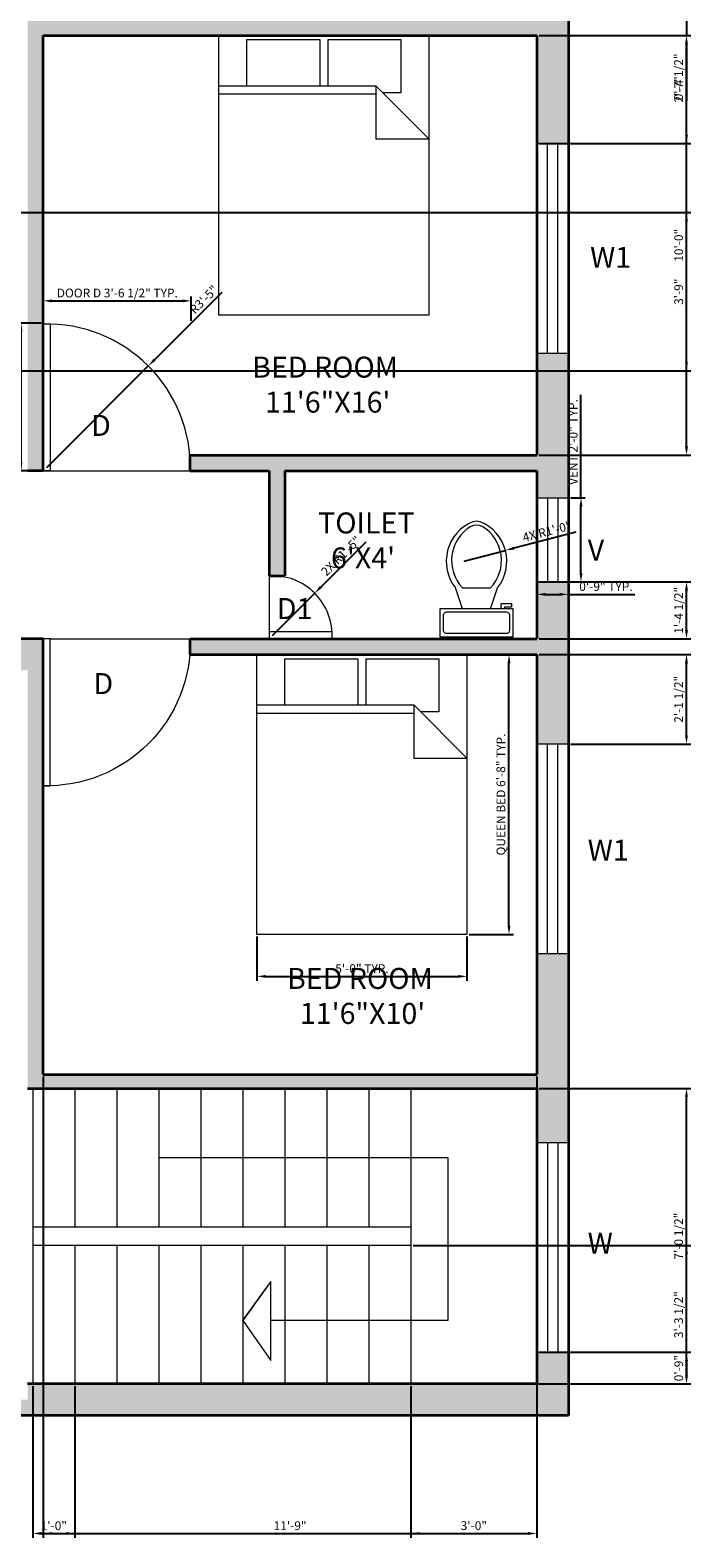
# Model space of a CAD drawing. Units: inches. Extents: x 5030 to 5465, y 5339 to 6047.
# Tile 2 of 5: x 5275 to 5465, y 5340 to 5771. Entities that reach past the tile are written whole.
import ezdxf

# ---------------------------------------------------------------- set-up
doc = ezdxf.new("R2010")
doc.units = ezdxf.units.IN
for name, color, linetype, lineweight in [('A-ANNO-DIMS', 2, 'Continuous', 18), ('A-ANNO-TEXT', 7, 'Continuous', 18), ('A-AREA-IDEN', 7, 'Continuous', 25), ('A-DOOR', 3, 'Continuous', 18), ('A-FLOR-FIXT', 9, 'Continuous', 18), ('A-FLOR-STRS', 7, 'Continuous', 18), ('A-FURN', 8, 'Continuous', 18), ('A-GLAZ', 4, 'Continuous', 18), ('A-WALL', 7, 'Continuous', 35)]:
    doc.layers.add(name, color=color, linetype=linetype, lineweight=lineweight)
doc.layers.add('A-WALL-PATT', color=149, linetype='Continuous', lineweight=13, true_color=0x444546)
doc.styles.get("Standard").update_dxf_attribs({"font": 'arial.ttf'})
doc.dimstyles.new('ISO-25', dxfattribs={"dimtxt": 2.5, "dimasz": 2.5, "dimexe": 1.25, "dimexo": 0.625, "dimtad": 1, "dimlunit": 3, "dimtxsty": 'Standard', "dimcen": 2.5, "dimadec": 0, "dimazin": 0, "dimtfac": 1, "dimtmove": 0, "dimatfit": 3, "dimfxl": 1, "dimarcsym": 0})

# ---------------------------------------------------------------- blocks, each defined once
blk = doc.blocks.new('Bed - Queen')
for p, q in [((0, -80.00003), (0, 0)), ((0, 0), (59.99999, 0)), ((59.99999, 0), (59.99999, -80.00003)), ((7.99999, -1.2), (28.79998, -1.2)), ((7.99999, -14.4), (7.99999, -1.2)), ((28.79998, -1.2), (28.79998, -14.4)), ((31.19999, -1.2), (51.99999, -1.2)), ((31.19999, -14.4), (31.19999, -1.2)), ((51.99999, -1.2), (51.99999, -16.4)), ((0, -14.4), (44.8, -14.4)), ((44.8, -16.8), (0, -16.8)), ((59.99999, -29.6), (44.8, -14.4)), ((44.8, -14.4), (44.8, -29.6)), ((51.99999, -16.4), (46.79936, -16.4)), ((44.8, -29.6), (59.99999, -29.6)), ((59.99999, -80.00003), (0, -80.00003))]:
    blk.add_line(p, q)
blk = doc.blocks.new('Toilet - top')
for p, q in [((9.5, -6), (9.5, -2)), ((-10, -8.5), (-8, -8.5)), ((-10, -9.5), (-10, -8.5)), ((-8, -8.5), (-8, -8)), ((-7, -8), (-7, -9.5)), ((-4, -8), (-6, -14)), ((4, -8), (6, -14)), ((-7, -9.5), (-10, -9.5)), ((4, -14), (-4, -14))]:
    blk.add_line(p, q)
blk.add_lwpolyline([(10.5, -8), (10.5, 0), (-10.5, 0), (-10.5, -8)], close=True)
for points in [[(-9.5, -2), (-9.5, -6)], [(8.5, -1), (-8.5, -1)], [(-8.5, -7), (8.5, -7)]]:
    blk.add_lwpolyline(points)
for centre, radius, start, end in [((-8.62, -1.88), 0.884, 81.8699, 188.1301), ((8.62, -1.88), 0.884, 351.8699, 98.1301), ((-8.62, -6.12), 0.884, 171.8699, 278.1301), ((8.62, -6.12), 0.884, 261.8699, 8.1301), ((3.52, -21.58), 12.17, 141.4691, 247.9714), ((4.2, -21.82), 11.33, 136.3677, 238.9468), ((-3.52, -21.58), 12.17, 292.0284, 38.5307), ((-4.2, -21.82), 11.33, 301.053, 43.6321), ((0, -27.88), 4, 245.7318, 294.2682), ((0, -29), 4, 254.8605, 285.1395)]:
    blk.add_arc(centre, radius, start, end)
blk = doc.blocks.new('WIN-60IN')
for p, q in [((0, 60), (9, 60)), ((3, 60), (3, 0)), ((6, 60), (6, 0)), ((0, 0), (9, 0))]:
    blk.add_line(p, q)
blk = doc.blocks.new('VENT-24IN')
for p, q in [((0, 24), (9, 24)), ((3, 24), (3, 0)), ((6, 24), (6, 0)), ((0, 0), (9, 0))]:
    blk.add_line(p, q)
blk = doc.blocks.new('DOOR-SWING-42IN')
for p, q in [((0, 0), (0, 42)), ((0, 42), (2, 42)), ((2, 42), (2, 0)), ((2, 0), (0, 0))]:
    blk.add_line(p, q)
blk.add_arc((1, 1), 41.01, 358.6028, 91.3972)
blk = doc.blocks.new('DOOR-SWING-18IN')
for p, q in [((0, 18), (0, 2)), ((18, 2), (0, 2)), ((0, 2), (0, 0)), ((0, 0), (18, 0)), ((18, 0), (18, 2))]:
    blk.add_line(p, q)
blk.add_arc((1, 1), 17.03, 356.6335, 93.3665)
blk = doc.blocks.new('*D15')
at = {"layer": 'A-ANNO-DIMS', "color": 0, "lineweight": -2, "transparency": 16777216}
for p, q in [((5400.91, 5592), (5413.53, 5592)), ((5412.28, 5514.5), (5412.28, 5589.5)), ((5400.91, 5512), (5413.53, 5512))]:
    blk.add_line(p, q, dxfattribs=at)
at = {"layer": 'A-ANNO-DIMS', "color": 0, "transparency": 16777216}
for points in [[(5411.87, 5589.5), (5412.7, 5589.5), (5412.28, 5592)], [(5411.87, 5514.5), (5412.7, 5514.5), (5412.28, 5512)]]:
    blk.add_solid(points, dxfattribs=at)
at = {"layer": 'Defpoints', "color": 0, "transparency": 16777216}
for p in [(5400.28, 5592), (5412.28, 5592), (5400.28, 5512)]:
    blk.add_point(p, dxfattribs=at)
at = {"layer": 'A-ANNO-DIMS', "color": 0, "transparency": 16777216, "insert": (5410.29, 5552), "char_height": 2.5, "attachment_point": 5, "rotation": 90}
blk.add_mtext('QUEEN BED 6\'-8" TYP.', dxfattribs=at)
blk = doc.blocks.new('*D16')
at = {"layer": 'A-ANNO-DIMS', "color": 0, "lineweight": -2, "transparency": 16777216}
for p, q in [((5340.28, 5511.38), (5340.28, 5498.75)), ((5400.28, 5511.38), (5400.28, 5498.75)), ((5342.78, 5500), (5397.78, 5500))]:
    blk.add_line(p, q, dxfattribs=at)
at = {"layer": 'A-ANNO-DIMS', "color": 0, "transparency": 16777216}
for points in [[(5342.78, 5500.42), (5342.78, 5499.59), (5340.28, 5500)], [(5397.78, 5500.42), (5397.78, 5499.59), (5400.28, 5500)]]:
    blk.add_solid(points, dxfattribs=at)
at = {"layer": 'Defpoints', "color": 0, "transparency": 16777216}
for p in [(5340.28, 5512), (5400.28, 5512), (5400.28, 5500)]:
    blk.add_point(p, dxfattribs=at)
at = {"layer": 'A-ANNO-DIMS', "color": 0, "transparency": 16777216, "insert": (5370.28, 5501.9), "char_height": 2.5, "attachment_point": 5}
blk.add_mtext('5\'-0" TYP.', dxfattribs=at)
blk = doc.blocks.new('*D17')
at = {"layer": 'A-ANNO-DIMS', "color": 0, "lineweight": -2, "transparency": 16777216}
for p, q in [((5279.24, 5687.4), (5279.24, 5694.37)), ((5321.51, 5687.4), (5321.51, 5694.37)), ((5281.74, 5693.12), (5319.01, 5693.12))]:
    blk.add_line(p, q, dxfattribs=at)
at = {"layer": 'A-ANNO-DIMS', "color": 0, "transparency": 16777216}
for points in [[(5281.74, 5693.53), (5281.74, 5692.7), (5279.24, 5693.12)], [(5319.01, 5693.53), (5319.01, 5692.7), (5321.51, 5693.12)]]:
    blk.add_solid(points, dxfattribs=at)
at = {"layer": 'Defpoints', "color": 0, "transparency": 16777216}
for p in [(5321.51, 5693.12), (5279.24, 5686.78), (5321.51, 5686.78)]:
    blk.add_point(p, dxfattribs=at)
at = {"layer": 'A-ANNO-DIMS', "color": 0, "transparency": 16777216, "insert": (5300.38, 5695.04), "char_height": 2.5, "attachment_point": 5}
blk.add_mtext('DOOR D 3\'-6 1/2" TYP.', dxfattribs=at)
blk = doc.blocks.new('*D18')
at = {"layer": 'A-ANNO-DIMS', "color": 0, "lineweight": -2, "transparency": 16777216}
for p, q in [((5278.62, 5686.78), (5271.65, 5686.78)), ((5272.9, 5647), (5272.9, 5684.28)), ((5278.62, 5644.5), (5271.65, 5644.5))]:
    blk.add_line(p, q, dxfattribs=at)
at = {"layer": 'A-ANNO-DIMS', "color": 0, "transparency": 16777216}
for points in [[(5272.48, 5684.28), (5273.32, 5684.28), (5272.9, 5686.78)], [(5272.48, 5647), (5273.32, 5647), (5272.9, 5644.5)]]:
    blk.add_solid(points, dxfattribs=at)
at = {"layer": 'Defpoints', "color": 0, "transparency": 16777216}
for p in [(5272.9, 5686.78), (5279.24, 5686.78), (5279.24, 5644.5)]:
    blk.add_point(p, dxfattribs=at)
at = {"layer": 'A-ANNO-DIMS', "color": 0, "transparency": 16777216, "insert": (5270.98, 5665.64), "char_height": 2.5, "attachment_point": 5, "rotation": 90}
blk.add_mtext('3\'-6 1/2" TYP.', dxfattribs=at)
blk = doc.blocks.new('*D23')
at = {"layer": 'A-ANNO-DIMS', "color": 0, "lineweight": -2, "transparency": 16777216}
for p, q in [((5432.84, 5636.81), (5432.84, 5666.21)), ((5429.87, 5636.81), (5434.09, 5636.81)), ((5432.84, 5615.31), (5432.84, 5634.31)), ((5429.87, 5612.81), (5434.09, 5612.81))]:
    blk.add_line(p, q, dxfattribs=at)
at = {"layer": 'A-ANNO-DIMS', "color": 0, "transparency": 16777216}
for points in [[(5432.42, 5634.31), (5433.26, 5634.31), (5432.84, 5636.81)], [(5432.42, 5615.31), (5433.26, 5615.31), (5432.84, 5612.81)]]:
    blk.add_solid(points, dxfattribs=at)
at = {"layer": 'Defpoints', "color": 0, "transparency": 16777216}
for p in [(5429.24, 5636.81), (5432.84, 5636.81), (5429.24, 5612.81)]:
    blk.add_point(p, dxfattribs=at)
at = {"layer": 'A-ANNO-DIMS', "color": 0, "transparency": 16777216, "insert": (5430.94, 5652.76), "char_height": 2.5, "attachment_point": 5, "rotation": 90}
blk.add_mtext('VENT 2\'-0" TYP.', dxfattribs=at)
blk = doc.blocks.new('*D24')
at = {"layer": 'A-ANNO-DIMS', "color": 0, "lineweight": -2, "transparency": 16777216}
for p, q in [((5420.24, 5612.18), (5420.24, 5607.96)), ((5429.24, 5612.18), (5429.24, 5607.96)), ((5422.74, 5609.21), (5426.74, 5609.21)), ((5429.24, 5609.21), (5448.23, 5609.21))]:
    blk.add_line(p, q, dxfattribs=at)
at = {"layer": 'A-ANNO-DIMS', "color": 0, "transparency": 16777216}
for points in [[(5422.74, 5609.62), (5422.74, 5608.79), (5420.24, 5609.21)], [(5426.74, 5609.62), (5426.74, 5608.79), (5429.24, 5609.21)]]:
    blk.add_solid(points, dxfattribs=at)
at = {"layer": 'Defpoints', "color": 0, "transparency": 16777216}
for p in [(5420.24, 5612.81), (5429.24, 5612.81), (5429.24, 5609.21)]:
    blk.add_point(p, dxfattribs=at)
at = {"layer": 'A-ANNO-DIMS', "color": 0, "transparency": 16777216, "insert": (5439.98, 5611.11), "char_height": 2.5, "attachment_point": 5}
blk.add_mtext('0\'-9" TYP.', dxfattribs=at)
blk = doc.blocks.new('*D36')
at = {"layer": 'A-ANNO-DIMS', "color": 0, "lineweight": -2, "transparency": 16777216}
for p, q in [((5279.24, 5471.38), (5279.24, 5339.5)), ((5420.24, 5471.38), (5420.24, 5339.5)), ((5281.74, 5340.75), (5417.74, 5340.75))]:
    blk.add_line(p, q, dxfattribs=at)
at = {"layer": 'A-ANNO-DIMS', "color": 0, "transparency": 16777216}
for points in [[(5281.74, 5341.17), (5281.74, 5340.34), (5279.24, 5340.75)], [(5417.74, 5341.17), (5417.74, 5340.34), (5420.24, 5340.75)]]:
    blk.add_solid(points, dxfattribs=at)
at = {"layer": 'Defpoints', "color": 0, "transparency": 16777216}
for p in [(5279.24, 5472), (5420.24, 5472), (5420.24, 5340.75)]:
    blk.add_point(p, dxfattribs=at)
at = {"layer": 'A-ANNO-DIMS', "color": 0, "transparency": 16777216, "insert": (5349.74, 5342.65), "char_height": 2.5, "attachment_point": 5}
blk.add_mtext('11\'-9"', dxfattribs=at)
blk = doc.blocks.new('*D37')
at = {"layer": 'A-ANNO-DIMS', "color": 0, "lineweight": -2, "transparency": 16777216}
for p, q in [((5420.87, 5769), (5464.24, 5769)), ((5462.99, 5651.5), (5462.99, 5766.5)), ((5420.87, 5649), (5464.24, 5649))]:
    blk.add_line(p, q, dxfattribs=at)
at = {"layer": 'A-ANNO-DIMS', "color": 0, "transparency": 16777216}
for points in [[(5462.57, 5766.5), (5463.41, 5766.5), (5462.99, 5769)], [(5462.57, 5651.5), (5463.41, 5651.5), (5462.99, 5649)]]:
    blk.add_solid(points, dxfattribs=at)
at = {"layer": 'Defpoints', "color": 0, "transparency": 16777216}
for p in [(5420.24, 5769), (5462.99, 5769), (5420.24, 5649)]:
    blk.add_point(p, dxfattribs=at)
at = {"layer": 'A-ANNO-DIMS', "color": 0, "transparency": 16777216, "insert": (5461.09, 5709), "char_height": 2.5, "attachment_point": 5, "rotation": 90}
blk.add_mtext('10\'-0"', dxfattribs=at)
blk = doc.blocks.new('*D39')
at = {"layer": 'A-ANNO-DIMS', "color": 0, "lineweight": -2, "transparency": 16777216}
for p, q in [((5420.87, 5468), (5464.24, 5468)), ((5462.99, 5386), (5462.99, 5465.5)), ((5420.87, 5383.5), (5464.24, 5383.5))]:
    blk.add_line(p, q, dxfattribs=at)
at = {"layer": 'A-ANNO-DIMS', "color": 0, "transparency": 16777216}
for points in [[(5462.57, 5465.5), (5463.41, 5465.5), (5462.99, 5468)], [(5462.57, 5386), (5463.41, 5386), (5462.99, 5383.5)]]:
    blk.add_solid(points, dxfattribs=at)
at = {"layer": 'Defpoints', "color": 0, "transparency": 16777216}
for p in [(5420.24, 5468), (5462.99, 5468), (5420.24, 5383.5)]:
    blk.add_point(p, dxfattribs=at)
at = {"layer": 'A-ANNO-DIMS', "color": 0, "transparency": 16777216, "insert": (5461.07, 5425.75), "char_height": 2.5, "attachment_point": 5, "rotation": 90}
blk.add_mtext('7\'-0 1/2"', dxfattribs=at)
blk = doc.blocks.new('*D40')
at = {"layer": 'A-ANNO-DIMS', "color": 0, "lineweight": -2, "transparency": 16777216}
for p, q in [((5276.24, 5382.88), (5276.24, 5339.5)), ((5288.24, 5382.88), (5288.24, 5339.5)), ((5278.74, 5340.75), (5285.74, 5340.75))]:
    blk.add_line(p, q, dxfattribs=at)
at = {"layer": 'A-ANNO-DIMS', "color": 0, "transparency": 16777216}
for points in [[(5278.74, 5341.17), (5278.74, 5340.34), (5276.24, 5340.75)], [(5285.74, 5341.17), (5285.74, 5340.34), (5288.24, 5340.75)]]:
    blk.add_solid(points, dxfattribs=at)
at = {"layer": 'Defpoints', "color": 0, "transparency": 16777216}
for p in [(5276.24, 5383.5), (5288.24, 5383.5), (5288.24, 5340.75)]:
    blk.add_point(p, dxfattribs=at)
at = {"layer": 'A-ANNO-DIMS', "color": 0, "transparency": 16777216, "insert": (5282.24, 5342.65), "char_height": 2.5, "attachment_point": 5}
blk.add_mtext('1\'-0"', dxfattribs=at)
blk = doc.blocks.new('*D41')
at = {"layer": 'A-ANNO-DIMS', "color": 0, "lineweight": -2, "transparency": 16777216}
for p, q in [((5384.87, 5423.1), (5464.24, 5423.1)), ((5462.99, 5386), (5462.99, 5420.6)), ((5384.87, 5383.5), (5464.24, 5383.5))]:
    blk.add_line(p, q, dxfattribs=at)
at = {"layer": 'A-ANNO-DIMS', "color": 0, "transparency": 16777216}
for points in [[(5462.57, 5420.6), (5463.41, 5420.6), (5462.99, 5423.1)], [(5462.57, 5386), (5463.41, 5386), (5462.99, 5383.5)]]:
    blk.add_solid(points, dxfattribs=at)
at = {"layer": 'Defpoints', "color": 0, "transparency": 16777216}
for p in [(5384.24, 5423.1), (5462.99, 5423.1), (5384.24, 5383.5)]:
    blk.add_point(p, dxfattribs=at)
at = {"layer": 'A-ANNO-DIMS', "color": 0, "transparency": 16777216, "insert": (5461.07, 5403.3), "char_height": 2.5, "attachment_point": 5, "rotation": 90}
blk.add_mtext('3\'-3 1/2"', dxfattribs=at)
blk = doc.blocks.new('*D44')
at = {"layer": 'A-ANNO-DIMS', "color": 0, "lineweight": -2, "transparency": 16777216}
for p, q in [((5420.87, 5769), (5464.24, 5769)), ((5462.99, 5740.6), (5462.99, 5766.5)), ((5420.87, 5738.1), (5464.24, 5738.1))]:
    blk.add_line(p, q, dxfattribs=at)
at = {"layer": 'A-ANNO-DIMS', "color": 0, "transparency": 16777216}
for points in [[(5462.57, 5766.5), (5463.41, 5766.5), (5462.99, 5769)], [(5462.57, 5740.6), (5463.41, 5740.6), (5462.99, 5738.1)]]:
    blk.add_solid(points, dxfattribs=at)
at = {"layer": 'Defpoints', "color": 0, "transparency": 16777216}
for p in [(5420.24, 5769), (5462.99, 5769), (5420.24, 5738.1)]:
    blk.add_point(p, dxfattribs=at)
at = {"layer": 'A-ANNO-DIMS', "color": 0, "transparency": 16777216, "insert": (5461.11, 5753.55), "char_height": 2.5, "attachment_point": 5, "rotation": 90}
blk.add_mtext('2\'-7"', dxfattribs=at)
blk = doc.blocks.new('*D45')
at = {"layer": 'A-ANNO-DIMS', "color": 0, "lineweight": -2, "transparency": 16777216}
for p, q in [((5420.87, 5592), (5464.24, 5592)), ((5462.99, 5568.93), (5462.99, 5589.5)), ((5429.87, 5566.43), (5464.24, 5566.43))]:
    blk.add_line(p, q, dxfattribs=at)
at = {"layer": 'A-ANNO-DIMS', "color": 0, "transparency": 16777216}
for points in [[(5462.57, 5589.5), (5463.41, 5589.5), (5462.99, 5592)], [(5462.57, 5568.93), (5463.41, 5568.93), (5462.99, 5566.43)]]:
    blk.add_solid(points, dxfattribs=at)
at = {"layer": 'Defpoints', "color": 0, "transparency": 16777216}
for p in [(5420.24, 5592), (5462.99, 5592), (5429.24, 5566.43)]:
    blk.add_point(p, dxfattribs=at)
at = {"layer": 'A-ANNO-DIMS', "color": 0, "transparency": 16777216, "insert": (5461.07, 5579.22), "char_height": 2.5, "attachment_point": 5, "rotation": 90}
blk.add_mtext('2\'-1 1/2"', dxfattribs=at)
blk = doc.blocks.new('*D46')
at = {"layer": 'A-ANNO-DIMS', "color": 0, "lineweight": -2, "transparency": 16777216}
for p, q in [((5420.87, 5392.54), (5464.24, 5392.54)), ((5462.99, 5390.04), (5462.99, 5386)), ((5420.87, 5383.5), (5464.24, 5383.5))]:
    blk.add_line(p, q, dxfattribs=at)
at = {"layer": 'A-ANNO-DIMS', "color": 0, "transparency": 16777216}
for points in [[(5462.57, 5390.04), (5463.41, 5390.04), (5462.99, 5392.54)], [(5462.57, 5386), (5463.41, 5386), (5462.99, 5383.5)]]:
    blk.add_solid(points, dxfattribs=at)
at = {"layer": 'Defpoints', "color": 0, "transparency": 16777216}
for p in [(5420.24, 5392.54), (5420.24, 5383.5), (5462.99, 5383.5)]:
    blk.add_point(p, dxfattribs=at)
at = {"layer": 'A-ANNO-DIMS', "color": 0, "transparency": 16777216, "insert": (5461.09, 5388.02), "char_height": 2.5, "attachment_point": 5, "rotation": 90}
blk.add_mtext('0\'-9"', dxfattribs=at)
blk = doc.blocks.new('*D51')
at = {"layer": 'A-ANNO-DIMS', "color": 0, "lineweight": -2, "transparency": 16777216}
for p, q in [((5420.87, 5612.81), (5464.24, 5612.81)), ((5462.99, 5599), (5462.99, 5610.31)), ((5420.87, 5596.5), (5464.24, 5596.5))]:
    blk.add_line(p, q, dxfattribs=at)
at = {"layer": 'A-ANNO-DIMS', "color": 0, "transparency": 16777216}
for points in [[(5462.57, 5610.31), (5463.41, 5610.31), (5462.99, 5612.81)], [(5462.57, 5599), (5463.41, 5599), (5462.99, 5596.5)]]:
    blk.add_solid(points, dxfattribs=at)
at = {"layer": 'Defpoints', "color": 0, "transparency": 16777216}
for p in [(5420.24, 5612.81), (5462.99, 5612.81), (5420.24, 5596.5)]:
    blk.add_point(p, dxfattribs=at)
at = {"layer": 'A-ANNO-DIMS', "color": 0, "transparency": 16777216, "insert": (5461.07, 5604.66), "char_height": 2.5, "attachment_point": 5, "rotation": 90}
blk.add_mtext('1\'-4 1/2"', dxfattribs=at)
blk = doc.blocks.new('*D59')
at = {"layer": 'A-ANNO-DIMS', "color": 0, "lineweight": -2, "transparency": 16777216}
for p, q in [((5173.08, 5718.33), (5464.24, 5718.33)), ((5462.99, 5675.62), (5462.99, 5715.83)), ((5173.08, 5673.12), (5464.24, 5673.12))]:
    blk.add_line(p, q, dxfattribs=at)
at = {"layer": 'A-ANNO-DIMS', "color": 0, "transparency": 16777216}
for points in [[(5462.57, 5715.83), (5463.41, 5715.83), (5462.99, 5718.33)], [(5462.57, 5675.62), (5463.41, 5675.62), (5462.99, 5673.12)]]:
    blk.add_solid(points, dxfattribs=at)
at = {"layer": 'Defpoints', "color": 0, "transparency": 16777216}
for p in [(5172.45, 5718.33), (5462.99, 5718.33), (5172.45, 5673.12)]:
    blk.add_point(p, dxfattribs=at)
at = {"layer": 'A-ANNO-DIMS', "color": 0, "transparency": 16777216, "insert": (5461.09, 5695.72), "char_height": 2.5, "attachment_point": 5, "rotation": 90}
blk.add_mtext('3\'-9"', dxfattribs=at)
blk = doc.blocks.new('*D61')
at = {"layer": 'A-ANNO-DIMS', "color": 0, "lineweight": -2, "transparency": 16777216}
for p, q in [((5384.24, 5382.88), (5384.24, 5339.5)), ((5420.24, 5382.88), (5420.24, 5339.5)), ((5386.74, 5340.75), (5417.74, 5340.75))]:
    blk.add_line(p, q, dxfattribs=at)
at = {"layer": 'A-ANNO-DIMS', "color": 0, "transparency": 16777216}
for points in [[(5386.74, 5341.17), (5386.74, 5340.34), (5384.24, 5340.75)], [(5417.74, 5341.17), (5417.74, 5340.34), (5420.24, 5340.75)]]:
    blk.add_solid(points, dxfattribs=at)
at = {"layer": 'Defpoints', "color": 0, "transparency": 16777216}
for p in [(5384.24, 5383.5), (5420.24, 5383.5), (5420.24, 5340.75)]:
    blk.add_point(p, dxfattribs=at)
at = {"layer": 'A-ANNO-DIMS', "color": 0, "transparency": 16777216, "insert": (5402.24, 5342.66), "char_height": 2.5, "attachment_point": 5}
blk.add_mtext('3\'-0"', dxfattribs=at)
blk = doc.blocks.new('*D62')
at = {"layer": 'A-ANNO-DIMS', "color": 0, "lineweight": -2, "transparency": 16777216}
for p, q in [((5462.99, 5776), (5462.99, 5778.5)), ((5420.87, 5773.5), (5464.24, 5773.5)), ((5462.99, 5773.5), (5462.99, 5769)), ((5420.87, 5769), (5464.24, 5769)), ((5462.99, 5766.5), (5462.99, 5750.28))]:
    blk.add_line(p, q, dxfattribs=at)
at = {"layer": 'A-ANNO-DIMS', "color": 0, "transparency": 16777216}
for points in [[(5462.57, 5776), (5463.41, 5776), (5462.99, 5773.5)], [(5462.57, 5766.5), (5463.41, 5766.5), (5462.99, 5769)]]:
    blk.add_solid(points, dxfattribs=at)
at = {"layer": 'Defpoints', "color": 0, "transparency": 16777216}
for p in [(5420.24, 5773.5), (5420.24, 5769), (5462.99, 5769)]:
    blk.add_point(p, dxfattribs=at)
at = {"layer": 'A-ANNO-DIMS', "color": 0, "transparency": 16777216, "insert": (5461.07, 5757.14), "char_height": 2.5, "attachment_point": 5, "rotation": 90}
blk.add_mtext('0\'-4 1/2"', dxfattribs=at)
blk = doc.blocks.new('*D64')
at = {"layer": 'A-ANNO-DIMS', "color": 0, "lineweight": -2, "transparency": 16777216}
for p, q in [((5330.28, 5695.54), (5311.01, 5676.27)), ((5280.24, 5645.5), (5309.24, 5674.5))]:
    blk.add_line(p, q, dxfattribs=at)
at = {"layer": 'A-ANNO-DIMS', "color": 0, "transparency": 16777216}
blk.add_solid([(5310.71, 5676.57), (5311.3, 5675.98), (5309.24, 5674.5)], dxfattribs=at)
at = {"layer": 'Defpoints', "color": 0, "transparency": 16777216}
for p in [(5309.24, 5674.5), (5280.24, 5645.5)]:
    blk.add_point(p, dxfattribs=at)
at = {"layer": 'A-ANNO-DIMS', "color": 0, "transparency": 16777216, "insert": (5325.3, 5693.25), "char_height": 2.5, "attachment_point": 5, "rotation": 45.0001}
blk.add_mtext('R3\'-5"', dxfattribs=at)
blk = doc.blocks.new('*D65')
at = {"layer": 'A-ANNO-DIMS', "color": 0, "lineweight": -2, "transparency": 16777216}
for p, q in [((5371.42, 5624.18), (5358.55, 5611.31)), ((5344.74, 5597.5), (5356.78, 5609.54))]:
    blk.add_line(p, q, dxfattribs=at)
at = {"layer": 'A-ANNO-DIMS', "color": 0, "transparency": 16777216}
blk.add_solid([(5358.25, 5611.61), (5358.84, 5611.02), (5356.78, 5609.54)], dxfattribs=at)
at = {"layer": 'Defpoints', "color": 0, "transparency": 16777216}
for p in [(5356.78, 5609.54), (5344.74, 5597.5)]:
    blk.add_point(p, dxfattribs=at)
at = {"layer": 'A-ANNO-DIMS', "color": 0, "transparency": 16777216, "insert": (5364.52, 5619.98), "char_height": 2.5, "attachment_point": 5, "rotation": 45.0002}
blk.add_mtext('2X R1\'-5"', dxfattribs=at)
blk = doc.blocks.new('*D68')
at = {"layer": 'A-ANNO-DIMS', "color": 0, "lineweight": -2, "transparency": 16777216}
for p, q in [((5431.34, 5627.04), (5413.68, 5622.41)), ((5399.49, 5618.68), (5411.26, 5621.77))]:
    blk.add_line(p, q, dxfattribs=at)
at = {"layer": 'A-ANNO-DIMS', "color": 0, "transparency": 16777216}
blk.add_solid([(5413.57, 5622.81), (5413.78, 5622), (5411.26, 5621.77)], dxfattribs=at)
at = {"layer": 'Defpoints', "color": 0, "transparency": 16777216}
for p in [(5411.26, 5621.77), (5399.49, 5618.68)]:
    blk.add_point(p, dxfattribs=at)
at = {"layer": 'A-ANNO-DIMS', "color": 0, "transparency": 16777216, "insert": (5423.23, 5626.88), "char_height": 2.5, "attachment_point": 5, "rotation": 14.7177}
blk.add_mtext('4X R1\'-0"', dxfattribs=at)

msp = doc.modelspace()

# ---------------------------------------------------------------- hatches: boundary and pattern name
at = {"layer": 'A-WALL-PATT'}
h = msp.add_hatch(color=256, dxfattribs=at)
h.dxf.hatch_style = 1
h.paths.add_polyline_path([(5227.999, 5974.503), (5069.24, 5974.503), (5069.24, 5942.38), (5078.24, 5942.38), (5078.24, 5965.503), (5198.24, 5965.503), (5198.24, 5916.003), (5274.74, 5916.003), (5274.74, 5869.503), (5202.74, 5869.503), (5202.74, 5898.003), (5198.24, 5898.003), (5198.24, 5865.003), (5274.74, 5865.003), (5274.74, 5817.003, -0.0121933), (5276.74, 5817.003), (5279.24, 5817.003), (5279.24, 5947.503, -0.0293864), (5277.24, 5947.503), (5274.74, 5947.503), (5274.74, 5920.503), (5202.74, 5920.503), (5202.74, 5965.503), (5227.999, 5965.503)])
h.paths.add_polyline_path([(5078.24, 5894.38), (5069.24, 5894.38), (5069.24, 5845.837), (5078.24, 5845.837), (5078.24, 5865.003), (5138.24, 5865.003), (5138.24, 5869.503), (5078.24, 5869.503)], flags=17)
h.paths.add_polyline_path([(5316.341, 5974.503), (5251.999, 5974.503), (5251.999, 5965.503), (5279.24, 5965.503), (5316.341, 5965.503)])
h.paths.add_polyline_path([(5429.24, 5974.503), (5376.341, 5974.503), (5376.341, 5965.503), (5420.24, 5965.503), (5420.24, 5904.986), (5429.24, 5904.986)])
h.paths.add_polyline_path([(5429.24, 5844.986), (5420.24, 5844.986), (5420.24, 5773.503), (5279.24, 5773.503), (5279.24, 5775.003), (5274.74, 5775.003), (5274.74, 5644.503), (5279.24, 5644.503), (5279.24, 5686.503), (5279.24, 5769.003), (5420.24, 5769.003), (5420.24, 5738.095), (5429.24, 5738.095)])
h.paths.add_polyline_path([(5429.24, 5678.095), (5420.24, 5678.095), (5420.24, 5649.003), (5321.24, 5649.003), (5321.24, 5646.503, -0.0121933), (5321.24, 5644.503), (5343.74, 5644.503), (5343.74, 5614.503, -0.0293864), (5345.74, 5614.503), (5348.24, 5614.503), (5348.24, 5644.503), (5420.24, 5644.503), (5420.24, 5636.807), (5429.24, 5636.807)])
h.paths.add_polyline_path([(5429.24, 5612.807), (5420.24, 5612.807), (5420.24, 5596.503), (5321.24, 5596.503, -0.0121933), (5321.24, 5594.503), (5321.24, 5592.003), (5420.24, 5592.003), (5420.24, 5566.431), (5429.24, 5566.431)])
h.paths.add_polyline_path([(5429.24, 5506.431), (5420.24, 5506.431), (5420.24, 5472.003), (5279.24, 5472.003), (5279.24, 5596.503), (5126.24, 5596.503), (5126.24, 5589.503, -0.0106371), (5126.24, 5587.503), (5274.74, 5587.503), (5274.74, 5468.003), (5420.24, 5468.003), (5420.24, 5452.536), (5429.24, 5452.536)])
h.paths.add_polyline_path([(5429.24, 5392.536), (5420.24, 5392.536), (5420.24, 5383.503), (5274.74, 5383.503), (5274.74, 5374.503), (5429.24, 5374.503)])
h.paths.add_polyline_path([(5101.667, 5383.503), (5078.24, 5383.503), (5078.24, 5683.152), (5069.24, 5683.152), (5069.24, 5374.503), (5101.667, 5374.503)])
h.paths.add_polyline_path([(5078.24, 5770.503), (5221.745, 5770.503), (5221.745, 5775.003), (5078.24, 5775.003), (5078.24, 5785.837), (5069.24, 5785.837), (5069.24, 5743.152), (5078.24, 5743.152)])
h.paths.add_polyline_path([(5274.74, 5379.003), (5101.667, 5379.003), (5101.667, 5374.503), (5274.74, 5374.503)])

# ---------------------------------------------------------------- linework, layer by layer
at = {"layer": 'A-DOOR'}
for p, q in [((5279.24, 5644.503), (5321.24, 5644.503)), ((5279.24, 5596.503), (5279.24, 5596.503)), ((5281.24, 5596.503), (5321.24, 5596.503))]:
    msp.add_line(p, q, dxfattribs=at)
at = {"layer": 'A-FLOR-STRS'}
for p, q in [((5276.24, 5468.003), (5276.24, 5383.503)), ((5288.24, 5468.003), (5288.24, 5428.403)), ((5300.24, 5468.003), (5300.24, 5428.403)), ((5300.24, 5468.003), (5300.24, 5428.403)), ((5312.24, 5468.003), (5312.24, 5428.403)), ((5324.24, 5468.003), (5324.24, 5428.403)), ((5336.24, 5468.003), (5336.24, 5428.403)), ((5336.24, 5468.003), (5336.24, 5428.403)), ((5348.24, 5468.003), (5348.24, 5428.403)), ((5360.24, 5468.003), (5360.24, 5428.403)), ((5372.24, 5468.003), (5372.24, 5428.403)), ((5372.24, 5468.003), (5372.24, 5428.403)), ((5372.24, 5468.003), (5372.24, 5428.403)), ((5384.24, 5468.003), (5384.24, 5383.503)), ((5312.24, 5448.203), (5394.779, 5448.203)), ((5394.779, 5448.203), (5394.779, 5401.658)), ((5276.24, 5428.403), (5384.24, 5428.403)), ((5384.24, 5423.103), (5276.24, 5423.103)), ((5288.24, 5423.103), (5288.24, 5383.503)), ((5300.24, 5423.103), (5300.24, 5383.503)), ((5300.24, 5423.103), (5300.24, 5383.503)), ((5312.24, 5423.103), (5312.24, 5383.503)), ((5324.24, 5423.103), (5324.24, 5383.503)), ((5336.24, 5423.103), (5336.24, 5383.503)), ((5336.24, 5423.103), (5336.24, 5383.503)), ((5348.24, 5423.103), (5348.24, 5383.503)), ((5360.24, 5423.103), (5360.24, 5383.503)), ((5372.24, 5423.103), (5372.24, 5383.503)), ((5372.24, 5423.103), (5372.24, 5383.503)), ((5372.24, 5423.103), (5372.24, 5383.503)), ((5344.284, 5412.737), (5336.24, 5401.658)), ((5336.24, 5401.658), (5343.407, 5411.53)), ((5344.284, 5390.201), (5344.284, 5412.737)), ((5336.24, 5401.658), (5344.284, 5390.201)), ((5394.779, 5401.658), (5344.284, 5401.658))]:
    msp.add_line(p, q, dxfattribs=at)
at = {"layer": 'A-WALL'}
for p, q in [((5429.24, 5974.503), (5429.24, 5374.503)), ((5279.24, 5644.503), (5279.24, 5769.003)), ((5279.24, 5769.003), (5420.24, 5769.003)), ((5420.24, 5769.003), (5420.24, 5649.003)), ((5321.24, 5649.003), (5420.24, 5649.003)), ((5321.24, 5644.503), (5321.24, 5649.003)), ((5279.24, 5644.503), (5274.74, 5644.503)), ((5321.24, 5644.503), (5343.74, 5644.503)), ((5343.74, 5644.503), (5343.74, 5614.503)), ((5348.24, 5644.503), (5348.24, 5614.503)), ((5348.24, 5644.503), (5420.24, 5644.503)), ((5420.24, 5644.503), (5420.24, 5596.503)), ((5343.74, 5614.503), (5348.24, 5614.503)), ((5279.24, 5596.503), (5126.24, 5596.503)), ((5279.24, 5472.003), (5279.24, 5596.503)), ((5321.24, 5596.503), (5420.24, 5596.503)), ((5321.24, 5592.003), (5321.24, 5596.503)), ((5321.24, 5592.003), (5420.24, 5592.003)), ((5420.24, 5592.003), (5420.24, 5472.003)), ((5279.24, 5472.003), (5420.24, 5472.003)), ((5274.74, 5468.003), (5420.24, 5468.003)), ((5420.24, 5468.003), (5420.24, 5383.503)), ((5420.24, 5383.503), (5274.74, 5383.503)), ((5429.24, 5374.503), (5069.24, 5374.503))]:
    msp.add_line(p, q, dxfattribs=at)

# ---------------------------------------------------------------- block references
at = {"layer": 'A-DOOR'}
for name, p in [('DOOR-SWING-42IN', (5279.24, 5644.503)), ('DOOR-SWING-18IN', (5343.74, 5596.503))]:
    msp.add_blockref(name, p, dxfattribs=at)
at = {"layer": 'A-DOOR', "extrusion": (0, 0, -1), "zscale": -1, "rotation": 180}
msp.add_blockref('DOOR-SWING-42IN', (-5279.24, 5596.503), dxfattribs=at)
at = {"layer": 'A-FLOR-FIXT', "rotation": 180}
msp.add_blockref('Toilet - top', (5403.009, 5597.098), dxfattribs=at)
at = {"layer": 'A-FURN'}
for p in [(5329.401, 5769.003), (5340.285, 5592.003)]:
    msp.add_blockref('Bed - Queen', p, dxfattribs=at)
at = {"layer": 'A-GLAZ', "rotation": 180}
for p in [(5429.24, 5738.095), (5429.24, 5566.431)]:
    msp.add_blockref('WIN-60IN', p, dxfattribs=at)
at = {"layer": 'A-GLAZ'}
for name, p in [('VENT-24IN', (5420.24, 5612.807)), ('WIN-60IN', (5420.24, 5392.536))]:
    msp.add_blockref(name, p, dxfattribs=at)

# ---------------------------------------------------------------- texts
at = {"layer": 'A-ANNO-TEXT', "char_height": 6, "attachment_point": 1}
for s, insert in [('W1 ', (5435.448, 5708.561)), ('D', (5292.884, 5660.505)), ('V ', (5434.761, 5624.886)), ('D1 ', (5345.95, 5608.163)), ('D', (5293.577, 5586.711)), ('W1 ', (5434.761, 5539.085)), ('W ', (5434.761, 5426.728))]:
    msp.add_mtext_dynamic_manual_height_columns(s, width=54.21026, gutter_width=12.5, heights=[0], dxfattribs=dict(at, insert=insert))
at = {"layer": 'A-AREA-IDEN', "char_height": 6, "attachment_point": 1}
for s, insert in [(' BED ROOM\\P   11\'6"X16\'', (5337.074, 5677.174)), (" TOILET\\P   6'X4'", (5355.928, 5632.626)), (' {\\fTimes New Roman|b0|i0|c0|p18;BED ROOM\\P   11\'6"X10\'}', (5347.023, 5502.422))]:
    msp.add_mtext_dynamic_manual_height_columns(s, width=54.21026, gutter_width=12.5, heights=[0], dxfattribs=dict(at, insert=insert))

# ---------------------------------------------------------------- dimensions: what is measured, and where the dimension line sits
at = {"layer": 'A-ANNO-DIMS'}
for base, p1, p2, picture, middle in [((5462.99, 5769.003), (5420.24, 5773.503), (5420.24, 5769.003), '*D62', (5461.073, 5757.143)), ((5462.99, 5769.003), (5420.24, 5649.003), (5420.24, 5769.003), '*D37', (5461.089, 5709.003)), ((5462.99, 5769.003), (5420.24, 5738.095), (5420.24, 5769.003), '*D44', (5461.11, 5753.549)), ((5462.99, 5718.328), (5172.454, 5673.117), (5172.454, 5718.328), '*D59', (5461.088, 5695.723)), ((5462.99, 5612.807), (5420.24, 5596.503), (5420.24, 5612.807), '*D51', (5461.073, 5604.655)), ((5462.99, 5592.003), (5429.24, 5566.431), (5420.24, 5592.003), '*D45', (5461.073, 5579.217)), ((5462.99, 5468.003), (5420.24, 5383.503), (5420.24, 5468.003), '*D39', (5461.073, 5425.753)), ((5462.99, 5423.103), (5384.24, 5383.503), (5384.24, 5423.103), '*D41', (5461.072, 5403.303)), ((5462.99, 5383.503), (5420.24, 5392.536), (5420.24, 5383.503), '*D46', (5461.089, 5388.019))]:
    dim = msp.add_linear_dim(base=base, p1=p1, p2=p2, angle=90, dimstyle='ISO-25', override={"dimdec": 1, "dimlfac": 1, "dimrnd": 0, "dimzin": 1, "dimdsep": 46, "dimlunit": 4, "dimfrac": 2}, dxfattribs=at)
    dim.commit()
    dim.dimension.update_dxf_attribs({"geometry": picture, "text_midpoint": middle})
for base, p1, p2, text, picture, middle in [((5321.514, 5693.118), (5279.24, 5686.777), (5321.514, 5686.777), 'DOOR D <> TYP.', '*D17', (5300.377, 5695.037)), ((5429.24, 5609.207), (5420.24, 5612.807), (5429.24, 5612.807), '<> TYP.', '*D24', (5439.985, 5611.109)), ((5400.285, 5500.003), (5340.285, 5512.003), (5400.285, 5512.003), '<> TYP.', '*D16', (5370.285, 5501.905))]:
    dim = msp.add_linear_dim(base=base, p1=p1, p2=p2, text=text, dimstyle='ISO-25', override={"dimdec": 1, "dimlfac": 1, "dimrnd": 0, "dimzin": 1, "dimdsep": 46, "dimlunit": 4, "dimfrac": 2}, dxfattribs=at)
    dim.commit()
    dim.dimension.update_dxf_attribs({"geometry": picture, "text_midpoint": middle})
dim = msp.add_radius_dim(center=(5280.24, 5645.503), mpoint=(5309.24, 5674.503), dimstyle='ISO-25', override={"dimdec": 1, "dimlfac": 1, "dimrnd": 0, "dimzin": 1, "dimdsep": 46, "dimlunit": 4, "dimfrac": 2}, dxfattribs=at)
dim.commit()
dim.dimension.update_dxf_attribs({"geometry": '*D64', "text_midpoint": (5326.64, 5691.903), "dimtype": 164})
for base, p1, p2, text, picture, middle in [((5272.899, 5686.777), (5279.24, 5644.503), (5279.24, 5686.777), '<> TYP.', '*D18', (5270.981, 5665.64)), ((5432.84, 5636.807), (5429.24, 5612.807), (5429.24, 5636.807), 'VENT <> TYP.', '*D23', (5430.939, 5652.759)), ((5412.285, 5592.003), (5400.285, 5512.003), (5400.285, 5592.003), 'QUEEN BED <> TYP.', '*D15', (5410.29, 5552.003))]:
    dim = msp.add_linear_dim(base=base, p1=p1, p2=p2, angle=90, text=text, dimstyle='ISO-25', override={"dimdec": 1, "dimlfac": 1, "dimrnd": 0, "dimzin": 1, "dimdsep": 46, "dimlunit": 4, "dimfrac": 2}, dxfattribs=at)
    dim.commit()
    dim.dimension.update_dxf_attribs({"geometry": picture, "text_midpoint": middle})
for center, mpoint, text, picture, middle in [((5399.489, 5618.678), (5411.259, 5621.77), '4X <>', '*D68', (5423.233, 5626.881)), ((5344.74, 5597.503), (5356.782, 5609.545), '2X <>', '*D65', (5364.524, 5619.977))]:
    dim = msp.add_radius_dim(center=center, mpoint=mpoint, text=text, dimstyle='ISO-25', override={"dimdec": 1, "dimlfac": 1, "dimrnd": 0, "dimzin": 1, "dimdsep": 46, "dimlunit": 4, "dimfrac": 2}, dxfattribs=at)
    dim.commit()
    dim.dimension.update_dxf_attribs({"geometry": picture, "text_midpoint": middle})
for base, p1, p2, picture, middle in [((5420.24, 5340.753), (5279.24, 5472.003), (5420.24, 5472.003), '*D36', (5349.74, 5342.655)), ((5288.24, 5340.753), (5276.24, 5383.503), (5288.24, 5383.503), '*D40', (5282.24, 5342.655)), ((5420.24, 5340.753), (5384.24, 5383.503), (5420.24, 5383.503), '*D61', (5402.24, 5342.655))]:
    dim = msp.add_linear_dim(base=base, p1=p1, p2=p2, dimstyle='ISO-25', override={"dimdec": 1, "dimlfac": 1, "dimrnd": 0, "dimzin": 1, "dimdsep": 46, "dimlunit": 4, "dimfrac": 2}, dxfattribs=at)
    dim.commit()
    dim.dimension.update_dxf_attribs({"geometry": picture, "text_midpoint": middle})

doc.saveas('drawing.dxf')
